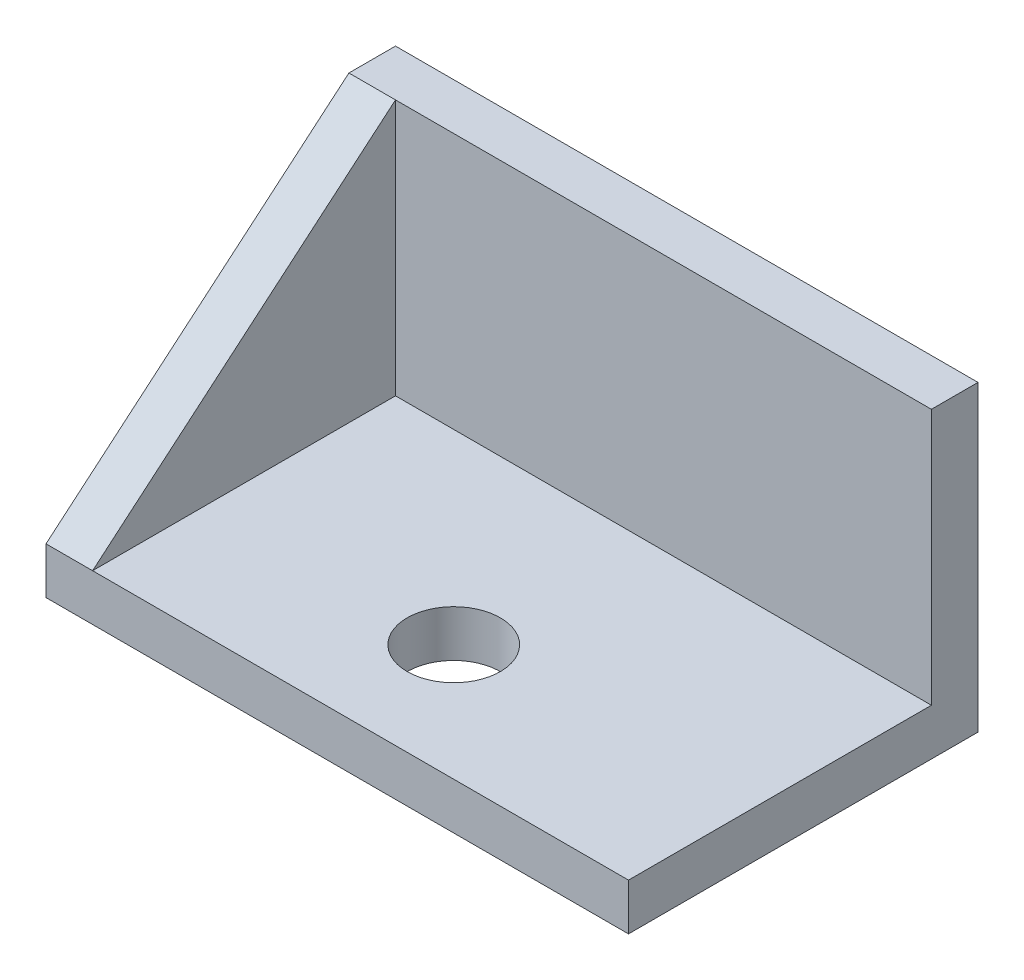
ISO-10303-21;
HEADER;
FILE_DESCRIPTION(('STEP AP214'),'2;1');
FILE_NAME('part.step','',(''),(''),'','','');
FILE_SCHEMA(('AUTOMOTIVE_DESIGN { 1 0 10303 214 1 1 1 1 }'));
ENDSEC;
DATA;
#1=APPLICATION_CONTEXT('core data for automotive mechanical design processes');
#2=APPLICATION_PROTOCOL_DEFINITION('international standard','automotive_design',2000,#1);
#3=PRODUCT_CONTEXT('',#1,'mechanical');
#4=PRODUCT('Part','Part','',(#3));
#5=PRODUCT_RELATED_PRODUCT_CATEGORY('part','',(#4));
#6=PRODUCT_DEFINITION_FORMATION('','',#4);
#7=PRODUCT_DEFINITION_CONTEXT('part definition',#1,'design');
#8=PRODUCT_DEFINITION('design','',#6,#7);
#9=PRODUCT_DEFINITION_SHAPE('','',#8);
#10=(LENGTH_UNIT() NAMED_UNIT(*) SI_UNIT(.MILLI.,.METRE.));
#11=(NAMED_UNIT(*) PLANE_ANGLE_UNIT() SI_UNIT($,.RADIAN.));
#12=(NAMED_UNIT(*) SI_UNIT($,.STERADIAN.) SOLID_ANGLE_UNIT());
#13=UNCERTAINTY_MEASURE_WITH_UNIT(LENGTH_MEASURE(1.E-05),#10,'distance_accuracy_value','');
#14=(GEOMETRIC_REPRESENTATION_CONTEXT(3) GLOBAL_UNCERTAINTY_ASSIGNED_CONTEXT((#13)) GLOBAL_UNIT_ASSIGNED_CONTEXT((#10,
#11,#12)) REPRESENTATION_CONTEXT('',''));
#15=CARTESIAN_POINT('',(0.,0.,0.));
#16=DIRECTION('',(0.,0.,1.));
#17=DIRECTION('',(1.,0.,0.));
#18=AXIS2_PLACEMENT_3D('',#15,#16,#17);
#19=CARTESIAN_POINT('',(0.,10.,75.));
#20=DIRECTION('',(0.,-1.,0.));
#21=DIRECTION('',(0.,0.,-1.));
#22=AXIS2_PLACEMENT_3D('',#19,#20,#21);
#23=PLANE('',#22);
#24=CARTESIAN_POINT('',(62.5,10.,50.));
#25=DIRECTION('',(0.,1.,0.));
#26=DIRECTION('',(0.,0.,1.));
#27=AXIS2_PLACEMENT_3D('',#24,#25,#26);
#28=CIRCLE('',#27,9.99999999999999);
#29=CARTESIAN_POINT('',(62.5,10.,60.));
#30=VERTEX_POINT('',#29);
#31=EDGE_CURVE('E180',#30,#30,#28,.T.);
#32=ORIENTED_EDGE('',*,*,#31,.F.);
#33=EDGE_LOOP('',(#32));
#34=FACE_BOUND('',#33,.T.);
#35=DIRECTION('',(0.,0.,-1.));
#36=VECTOR('',#35,1.);
#37=CARTESIAN_POINT('',(10.,10.,75.));
#38=LINE('',#37,#36);
#39=CARTESIAN_POINT('',(10.,10.,75.));
#40=VERTEX_POINT('',#39);
#41=CARTESIAN_POINT('',(10.,10.,10.));
#42=VERTEX_POINT('',#41);
#43=EDGE_CURVE('E141',#40,#42,#38,.T.);
#44=ORIENTED_EDGE('',*,*,#43,.F.);
#45=DIRECTION('',(-1.,0.,0.));
#46=VECTOR('',#45,1.);
#47=CARTESIAN_POINT('',(0.,10.,75.));
#48=LINE('',#47,#46);
#49=CARTESIAN_POINT('',(125.,10.,75.));
#50=VERTEX_POINT('',#49);
#51=EDGE_CURVE('E111',#50,#40,#48,.T.);
#52=ORIENTED_EDGE('',*,*,#51,.F.);
#53=DIRECTION('',(0.,0.,-1.));
#54=VECTOR('',#53,1.);
#55=CARTESIAN_POINT('',(125.,10.,75.));
#56=LINE('',#55,#54);
#57=CARTESIAN_POINT('',(125.,10.,9.99999999999999));
#58=VERTEX_POINT('',#57);
#59=EDGE_CURVE('E120',#50,#58,#56,.T.);
#60=ORIENTED_EDGE('',*,*,#59,.T.);
#61=DIRECTION('',(1.,0.,0.));
#62=VECTOR('',#61,1.);
#63=CARTESIAN_POINT('',(0.,10.,10.));
#64=LINE('',#63,#62);
#65=EDGE_CURVE('E135',#42,#58,#64,.T.);
#66=ORIENTED_EDGE('',*,*,#65,.F.);
#67=EDGE_LOOP('',(#44,#52,#60,#66));
#68=FACE_BOUND('',#67,.T.);
#69=ADVANCED_FACE('F39',(#34,#68),#23,.F.);
#70=CARTESIAN_POINT('',(0.,65.,10.));
#71=DIRECTION('',(0.,0.,-1.));
#72=DIRECTION('',(-1.,0.,0.));
#73=AXIS2_PLACEMENT_3D('',#70,#71,#72);
#74=PLANE('',#73);
#75=DIRECTION('',(0.,-1.,0.));
#76=VECTOR('',#75,1.);
#77=CARTESIAN_POINT('',(10.,65.,10.));
#78=LINE('',#77,#76);
#79=CARTESIAN_POINT('',(10.,65.,10.));
#80=VERTEX_POINT('',#79);
#81=EDGE_CURVE('E131',#80,#42,#78,.T.);
#82=ORIENTED_EDGE('',*,*,#81,.T.);
#83=ORIENTED_EDGE('',*,*,#65,.T.);
#84=DIRECTION('',(0.,-1.,0.));
#85=VECTOR('',#84,1.);
#86=CARTESIAN_POINT('',(125.,65.,9.99999999999999));
#87=LINE('',#86,#85);
#88=CARTESIAN_POINT('',(125.,65.,9.99999999999999));
#89=VERTEX_POINT('',#88);
#90=EDGE_CURVE('E110',#89,#58,#87,.T.);
#91=ORIENTED_EDGE('',*,*,#90,.F.);
#92=DIRECTION('',(1.,0.,0.));
#93=VECTOR('',#92,1.);
#94=CARTESIAN_POINT('',(0.,65.,10.));
#95=LINE('',#94,#93);
#96=EDGE_CURVE('E129',#80,#89,#95,.T.);
#97=ORIENTED_EDGE('',*,*,#96,.F.);
#98=EDGE_LOOP('',(#82,#83,#91,#97));
#99=FACE_BOUND('',#98,.T.);
#100=ADVANCED_FACE('F162',(#99),#74,.F.);
#101=CARTESIAN_POINT('',(0.,0.,75.));
#102=DIRECTION('',(1.,0.,0.));
#103=DIRECTION('',(0.,0.,-1.));
#104=AXIS2_PLACEMENT_3D('',#101,#102,#103);
#105=PLANE('',#104);
#106=DIRECTION('',(0.,-1.,0.));
#107=VECTOR('',#106,1.);
#108=CARTESIAN_POINT('',(0.,0.,75.));
#109=LINE('',#108,#107);
#110=CARTESIAN_POINT('',(0.,10.,75.));
#111=VERTEX_POINT('',#110);
#112=CARTESIAN_POINT('',(0.,0.,75.));
#113=VERTEX_POINT('',#112);
#114=EDGE_CURVE('E87',#111,#113,#109,.T.);
#115=ORIENTED_EDGE('',*,*,#114,.F.);
#116=DIRECTION('',(0.,0.645942241466174,-0.763386285369115));
#117=VECTOR('',#116,1.);
#118=CARTESIAN_POINT('',(0.,5.82758620689655,79.9310344827586));
#119=LINE('',#118,#117);
#120=CARTESIAN_POINT('',(0.,65.,10.));
#121=VERTEX_POINT('',#120);
#122=EDGE_CURVE('E146',#111,#121,#119,.T.);
#123=ORIENTED_EDGE('',*,*,#122,.T.);
#124=DIRECTION('',(0.,0.,1.));
#125=VECTOR('',#124,1.);
#126=CARTESIAN_POINT('',(0.,65.,0.));
#127=LINE('',#126,#125);
#128=CARTESIAN_POINT('',(0.,65.,0.));
#129=VERTEX_POINT('',#128);
#130=EDGE_CURVE('E106',#129,#121,#127,.T.);
#131=ORIENTED_EDGE('',*,*,#130,.F.);
#132=DIRECTION('',(0.,-1.,0.));
#133=VECTOR('',#132,1.);
#134=CARTESIAN_POINT('',(0.,0.,0.));
#135=LINE('',#134,#133);
#136=CARTESIAN_POINT('',(0.,0.,0.));
#137=VERTEX_POINT('',#136);
#138=EDGE_CURVE('E74',#129,#137,#135,.T.);
#139=ORIENTED_EDGE('',*,*,#138,.T.);
#140=DIRECTION('',(0.,0.,-1.));
#141=VECTOR('',#140,1.);
#142=CARTESIAN_POINT('',(0.,0.,75.));
#143=LINE('',#142,#141);
#144=EDGE_CURVE('E11',#113,#137,#143,.T.);
#145=ORIENTED_EDGE('',*,*,#144,.F.);
#146=EDGE_LOOP('',(#115,#123,#131,#139,#145));
#147=FACE_BOUND('',#146,.T.);
#148=ADVANCED_FACE('F41',(#147),#105,.F.);
#149=CARTESIAN_POINT('',(0.,0.,75.));
#150=DIRECTION('',(0.,1.,0.));
#151=DIRECTION('',(0.,0.,1.));
#152=AXIS2_PLACEMENT_3D('',#149,#150,#151);
#153=PLANE('',#152);
#154=CARTESIAN_POINT('',(62.5,0.,50.));
#155=DIRECTION('',(0.,1.,0.));
#156=DIRECTION('',(0.,0.,1.));
#157=AXIS2_PLACEMENT_3D('',#154,#155,#156);
#158=CIRCLE('',#157,9.99999999999999);
#159=CARTESIAN_POINT('',(62.5,0.,60.));
#160=VERTEX_POINT('',#159);
#161=EDGE_CURVE('E43',#160,#160,#158,.T.);
#162=ORIENTED_EDGE('',*,*,#161,.T.);
#163=EDGE_LOOP('',(#162));
#164=FACE_BOUND('',#163,.T.);
#165=DIRECTION('',(1.,0.,0.));
#166=VECTOR('',#165,1.);
#167=CARTESIAN_POINT('',(0.,0.,0.));
#168=LINE('',#167,#166);
#169=CARTESIAN_POINT('',(125.,0.,0.));
#170=VERTEX_POINT('',#169);
#171=EDGE_CURVE('E68',#137,#170,#168,.T.);
#172=ORIENTED_EDGE('',*,*,#171,.T.);
#173=DIRECTION('',(0.,0.,-1.));
#174=VECTOR('',#173,1.);
#175=CARTESIAN_POINT('',(125.,0.,75.));
#176=LINE('',#175,#174);
#177=CARTESIAN_POINT('',(125.,0.,75.));
#178=VERTEX_POINT('',#177);
#179=EDGE_CURVE('E47',#178,#170,#176,.T.);
#180=ORIENTED_EDGE('',*,*,#179,.F.);
#181=DIRECTION('',(1.,0.,0.));
#182=VECTOR('',#181,1.);
#183=CARTESIAN_POINT('',(0.,0.,75.));
#184=LINE('',#183,#182);
#185=EDGE_CURVE('E89',#113,#178,#184,.T.);
#186=ORIENTED_EDGE('',*,*,#185,.F.);
#187=ORIENTED_EDGE('',*,*,#144,.T.);
#188=EDGE_LOOP('',(#172,#180,#186,#187));
#189=FACE_BOUND('',#188,.T.);
#190=ADVANCED_FACE('F101',(#164,#189),#153,.F.);
#191=CARTESIAN_POINT('',(125.,0.,75.));
#192=DIRECTION('',(-1.,0.,0.));
#193=DIRECTION('',(0.,0.,1.));
#194=AXIS2_PLACEMENT_3D('',#191,#192,#193);
#195=PLANE('',#194);
#196=DIRECTION('',(0.,1.,0.));
#197=VECTOR('',#196,1.);
#198=CARTESIAN_POINT('',(125.,0.,0.));
#199=LINE('',#198,#197);
#200=CARTESIAN_POINT('',(125.,65.,0.));
#201=VERTEX_POINT('',#200);
#202=EDGE_CURVE('E98',#170,#201,#199,.T.);
#203=ORIENTED_EDGE('',*,*,#202,.T.);
#204=DIRECTION('',(0.,0.,-1.));
#205=VECTOR('',#204,1.);
#206=CARTESIAN_POINT('',(125.,65.,0.));
#207=LINE('',#206,#205);
#208=EDGE_CURVE('E130',#89,#201,#207,.T.);
#209=ORIENTED_EDGE('',*,*,#208,.F.);
#210=ORIENTED_EDGE('',*,*,#90,.T.);
#211=ORIENTED_EDGE('',*,*,#59,.F.);
#212=DIRECTION('',(0.,1.,0.));
#213=VECTOR('',#212,1.);
#214=CARTESIAN_POINT('',(125.,0.,75.));
#215=LINE('',#214,#213);
#216=EDGE_CURVE('E60',#178,#50,#215,.T.);
#217=ORIENTED_EDGE('',*,*,#216,.F.);
#218=ORIENTED_EDGE('',*,*,#179,.T.);
#219=EDGE_LOOP('',(#203,#209,#210,#211,#217,#218));
#220=FACE_BOUND('',#219,.T.);
#221=ADVANCED_FACE('F125',(#220),#195,.F.);
#222=CARTESIAN_POINT('',(0.,0.,75.));
#223=DIRECTION('',(0.,0.,-1.));
#224=DIRECTION('',(-1.,0.,0.));
#225=AXIS2_PLACEMENT_3D('',#222,#223,#224);
#226=PLANE('',#225);
#227=ORIENTED_EDGE('',*,*,#51,.T.);
#228=DIRECTION('',(1.,0.,0.));
#229=VECTOR('',#228,1.);
#230=CARTESIAN_POINT('',(-45.,10.,75.));
#231=LINE('',#230,#229);
#232=EDGE_CURVE('E94',#111,#40,#231,.T.);
#233=ORIENTED_EDGE('',*,*,#232,.F.);
#234=ORIENTED_EDGE('',*,*,#114,.T.);
#235=ORIENTED_EDGE('',*,*,#185,.T.);
#236=ORIENTED_EDGE('',*,*,#216,.T.);
#237=EDGE_LOOP('',(#227,#233,#234,#235,#236));
#238=FACE_BOUND('',#237,.T.);
#239=ADVANCED_FACE('F90',(#238),#226,.F.);
#240=CARTESIAN_POINT('',(0.,0.,0.));
#241=DIRECTION('',(0.,0.,-1.));
#242=DIRECTION('',(-1.,0.,0.));
#243=AXIS2_PLACEMENT_3D('',#240,#241,#242);
#244=PLANE('',#243);
#245=ORIENTED_EDGE('',*,*,#138,.F.);
#246=DIRECTION('',(-1.,0.,0.));
#247=VECTOR('',#246,1.);
#248=CARTESIAN_POINT('',(0.,65.,0.));
#249=LINE('',#248,#247);
#250=EDGE_CURVE('E112',#201,#129,#249,.T.);
#251=ORIENTED_EDGE('',*,*,#250,.F.);
#252=ORIENTED_EDGE('',*,*,#202,.F.);
#253=ORIENTED_EDGE('',*,*,#171,.F.);
#254=EDGE_LOOP('',(#245,#251,#252,#253));
#255=FACE_BOUND('',#254,.T.);
#256=ADVANCED_FACE('F124',(#255),#244,.T.);
#257=CARTESIAN_POINT('',(0.,65.,0.));
#258=DIRECTION('',(0.,1.,0.));
#259=DIRECTION('',(0.,0.,1.));
#260=AXIS2_PLACEMENT_3D('',#257,#258,#259);
#261=PLANE('',#260);
#262=DIRECTION('',(1.,0.,0.));
#263=VECTOR('',#262,1.);
#264=CARTESIAN_POINT('',(-45.,65.,10.));
#265=LINE('',#264,#263);
#266=EDGE_CURVE('E151',#121,#80,#265,.T.);
#267=ORIENTED_EDGE('',*,*,#266,.T.);
#268=ORIENTED_EDGE('',*,*,#96,.T.);
#269=ORIENTED_EDGE('',*,*,#208,.T.);
#270=ORIENTED_EDGE('',*,*,#250,.T.);
#271=ORIENTED_EDGE('',*,*,#130,.T.);
#272=EDGE_LOOP('',(#267,#268,#269,#270,#271));
#273=FACE_BOUND('',#272,.T.);
#274=ADVANCED_FACE('F157',(#273),#261,.T.);
#275=CARTESIAN_POINT('',(10.,65.,75.));
#276=DIRECTION('',(-1.,0.,0.));
#277=DIRECTION('',(0.,0.,1.));
#278=AXIS2_PLACEMENT_3D('',#275,#276,#277);
#279=PLANE('',#278);
#280=ORIENTED_EDGE('',*,*,#81,.F.);
#281=DIRECTION('',(0.,0.645942241466174,-0.763386285369114));
#282=VECTOR('',#281,1.);
#283=CARTESIAN_POINT('',(10.,65.,10.));
#284=LINE('',#283,#282);
#285=EDGE_CURVE('E170',#40,#80,#284,.T.);
#286=ORIENTED_EDGE('',*,*,#285,.F.);
#287=ORIENTED_EDGE('',*,*,#43,.T.);
#288=EDGE_LOOP('',(#280,#286,#287));
#289=FACE_BOUND('',#288,.T.);
#290=ADVANCED_FACE('F164',(#289),#279,.F.);
#291=CARTESIAN_POINT('',(-45.,65.,10.));
#292=DIRECTION('',(0.,-0.763386285369114,-0.645942241466174));
#293=DIRECTION('',(0.,0.645942241466174,-0.763386285369115));
#294=AXIS2_PLACEMENT_3D('',#291,#292,#293);
#295=PLANE('',#294);
#296=ORIENTED_EDGE('',*,*,#232,.T.);
#297=ORIENTED_EDGE('',*,*,#285,.T.);
#298=ORIENTED_EDGE('',*,*,#266,.F.);
#299=ORIENTED_EDGE('',*,*,#122,.F.);
#300=EDGE_LOOP('',(#296,#297,#298,#299));
#301=FACE_BOUND('',#300,.T.);
#302=ADVANCED_FACE('F175',(#301),#295,.F.);
#303=CARTESIAN_POINT('',(62.5,-45.,50.));
#304=DIRECTION('',(0.,1.,0.));
#305=DIRECTION('',(0.,0.,1.));
#306=AXIS2_PLACEMENT_3D('',#303,#304,#305);
#307=CYLINDRICAL_SURFACE('',#306,9.99999999999999);
#308=ORIENTED_EDGE('',*,*,#31,.T.);
#309=EDGE_LOOP('',(#308));
#310=FACE_BOUND('',#309,.T.);
#311=ORIENTED_EDGE('',*,*,#161,.F.);
#312=EDGE_LOOP('',(#311));
#313=FACE_BOUND('',#312,.T.);
#314=ADVANCED_FACE('F183',(#310,#313),#307,.F.);
#315=CLOSED_SHELL('',(#69,#100,#148,#190,#221,#239,#256,#274,#290,#302,#314));
#316=MANIFOLD_SOLID_BREP('B2',#315);
#317=ADVANCED_BREP_SHAPE_REPRESENTATION('',(#18,#316),#14);
#318=SHAPE_DEFINITION_REPRESENTATION(#9,#317);
ENDSEC;
END-ISO-10303-21;
